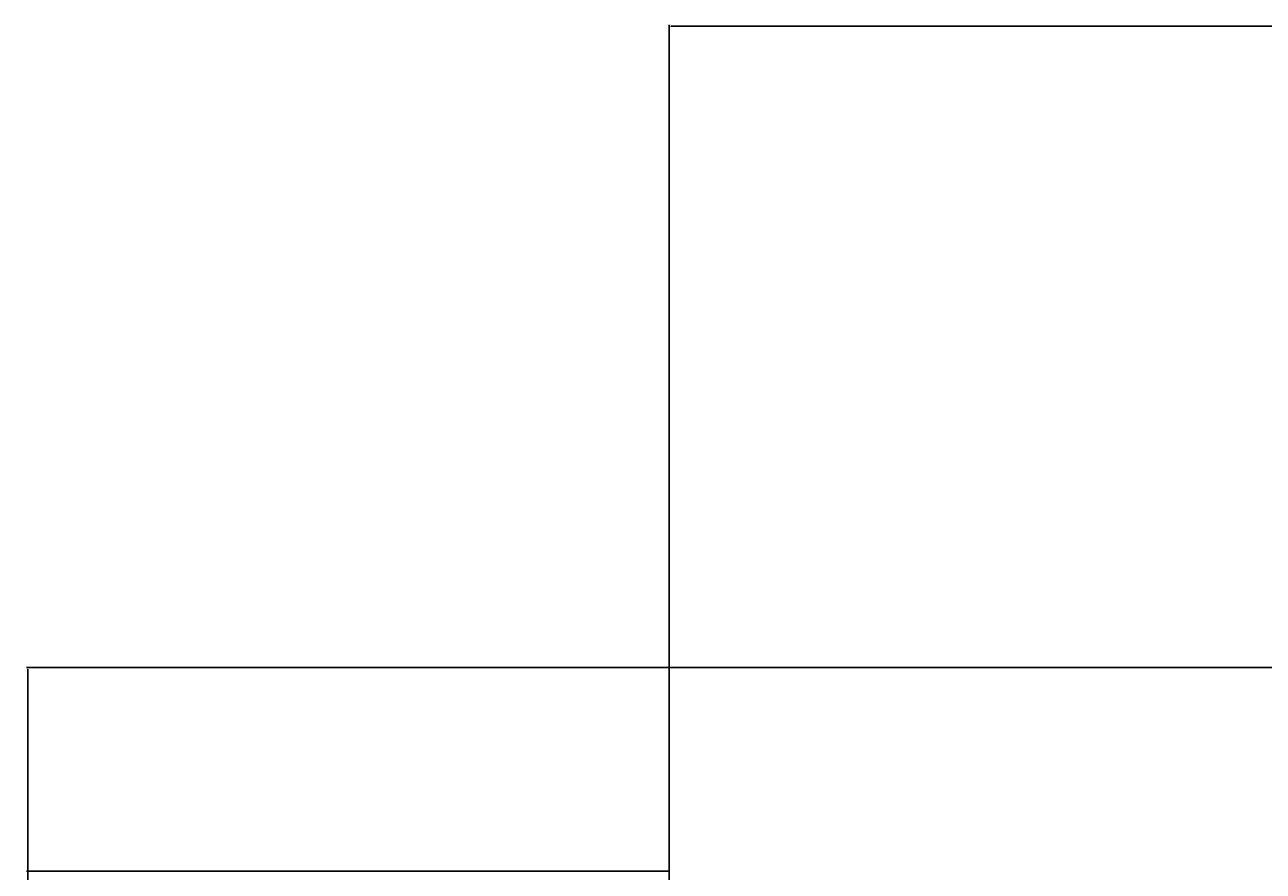
# Model space of a CAD drawing. Units: inches. Extents: x -61 to 1599, y -1316 to 257.
# Tile 113 of 204: x -61 to 85, y 158 to 257. Entities that reach past the tile are written whole.
import ezdxf

# ---------------------------------------------------------------- set-up
doc = ezdxf.new("R2010")
doc.units = ezdxf.units.IN
doc.header["$MEASUREMENT"] = 0
doc.layers.add('A-ANNO-DIMS', color=2, linetype='Continuous', lineweight=18)
doc.styles.get("Standard").update_dxf_attribs({"font": 'arial.ttf'})
doc.dimstyles.get("Standard").update_dxf_attribs({"dimtxt": 0.18, "dimasz": 0.18, "dimexe": 0.18, "dimexo": 0.0625, "dimgap": 0.09, "dimtad": 0, "dimtih": 1, "dimtoh": 1, "dimdec": 0, "dimzin": 0, "dimdsep": 46, "dimlunit": 3, "dimtxsty": 'Standard', "dimcen": 0.09, "dimadec": 0, "dimazin": 0, "dimtfac": 1, "dimtdec": 0, "dimtofl": 0, "dimtmove": 0, "dimatfit": 3, "dimfxl": 1, "dimtolj": 1, "dimtzin": 0, "dimarcsym": 0})

# ---------------------------------------------------------------- blocks, each defined once
blk = doc.blocks.new('*D686')
at = {"layer": 'A-ANNO-DIMS', "color": 0, "lineweight": -2, "transparency": 16777216}
for p, q in [((14.7, 157.74), (14.7, 257.46)), ((14.88, 257.28), (768.35, 257.28)), ((1522.52, 257.28), (769.05, 257.28)), ((1522.7, 157.74), (1522.7, 257.46))]:
    blk.add_line(p, q, dxfattribs=at)
at = {"layer": 'A-ANNO-DIMS', "color": 0, "transparency": 16777216}
for points in [[(14.88, 257.31), (14.88, 257.25), (14.7, 257.28)], [(1522.52, 257.31), (1522.52, 257.25), (1522.7, 257.28)]]:
    blk.add_solid(points, dxfattribs=at)
at = {"layer": 'DEFPOINTS', "color": 0, "transparency": 16777216}
for p in [(1522.7, 257.28), (14.7, 157.68), (1522.7, 157.68)]:
    blk.add_point(p, dxfattribs=at)
at = {"layer": 'A-ANNO-DIMS', "color": 0, "transparency": 16777216, "insert": (768.7, 257.28), "char_height": 0.18, "attachment_point": 5}
blk.add_mtext('\\A1;1508', dxfattribs=at)
blk = doc.blocks.new('*D687')
at = {"layer": 'A-ANNO-DIMS', "color": 0, "lineweight": -2, "transparency": 16777216}
for p, q in [((289.42, 181.68), (-61.08, 181.68)), ((-60.9, 181.5), (-60.9, -528.95)), ((-60.9, -1239.76), (-60.9, -529.32)), ((319.64, -1239.94), (-61.08, -1239.94))]:
    blk.add_line(p, q, dxfattribs=at)
at = {"layer": 'A-ANNO-DIMS', "color": 0, "transparency": 16777216}
for points in [[(-60.93, 181.5), (-60.87, 181.5), (-60.9, 181.68)], [(-60.93, -1239.76), (-60.87, -1239.76), (-60.9, -1239.94)]]:
    blk.add_solid(points, dxfattribs=at)
at = {"layer": 'DEFPOINTS', "color": 0, "transparency": 16777216}
for p in [(289.48, 181.68), (-60.9, -1239.94), (319.7, -1239.94)]:
    blk.add_point(p, dxfattribs=at)
at = {"layer": 'A-ANNO-DIMS', "color": 0, "transparency": 16777216, "insert": (-60.9, -529.13), "char_height": 0.18, "attachment_point": 5}
blk.add_mtext('\\A1;1421.6', dxfattribs=at)
blk = doc.blocks.new('*D691')
at = {"layer": 'A-ANNO-DIMS', "color": 0, "lineweight": -2, "transparency": 16777216}
for p, q in [((14.64, 157.68), (-61.08, 157.68)), ((-60.9, 157.5), (-60.9, -141.64)), ((-60.9, -441.14), (-60.9, -142)), ((14.64, -441.32), (-61.08, -441.32))]:
    blk.add_line(p, q, dxfattribs=at)
at = {"layer": 'A-ANNO-DIMS', "color": 0, "transparency": 16777216}
for points in [[(-60.93, 157.5), (-60.87, 157.5), (-60.9, 157.68)], [(-60.93, -441.14), (-60.87, -441.14), (-60.9, -441.32)]]:
    blk.add_solid(points, dxfattribs=at)
at = {"layer": 'DEFPOINTS', "color": 0, "transparency": 16777216}
for p in [(-60.9, 157.68), (14.7, 157.68), (14.7, -441.32)]:
    blk.add_point(p, dxfattribs=at)
at = {"layer": 'A-ANNO-DIMS', "color": 0, "transparency": 16777216, "insert": (-60.9, -141.82), "char_height": 0.18, "attachment_point": 5}
blk.add_mtext('\\A1;599', dxfattribs=at)
blk = doc.blocks.new('*D700')
at = {"layer": 'A-ANNO-DIMS', "color": 0, "lineweight": -2, "transparency": 16777216}
for p, q in [((14.7, -616.88), (14.7, 257.46)), ((14.88, 257.28), (96.77, 257.28)), ((179.57, 257.28), (97.68, 257.28)), ((179.75, -616.88), (179.75, 257.46))]:
    blk.add_line(p, q, dxfattribs=at)
at = {"layer": 'A-ANNO-DIMS', "color": 0, "transparency": 16777216}
for points in [[(14.88, 257.31), (14.88, 257.25), (14.7, 257.28)], [(179.57, 257.31), (179.57, 257.25), (179.75, 257.28)]]:
    blk.add_solid(points, dxfattribs=at)
at = {"layer": 'DEFPOINTS', "color": 0, "transparency": 16777216}
for p in [(179.75, 257.28), (14.7, -616.94), (179.75, -616.94)]:
    blk.add_point(p, dxfattribs=at)
at = {"layer": 'A-ANNO-DIMS', "color": 0, "transparency": 16777216, "insert": (97.23, 257.28), "char_height": 0.18, "attachment_point": 5}
blk.add_mtext('\\A1;165.05', dxfattribs=at)

msp = doc.modelspace()

# ---------------------------------------------------------------- dimensions: what is measured, and where the dimension line sits
at = {"layer": 'A-ANNO-DIMS'}
for base, p1, p2, override, picture, middle in [((1522.7028, 257.2771), (14.7028, 157.6771), (1522.7028, 157.6771), {"dimdec": 0, "dimlfac": 1, "dimrnd": 0, "dimzin": 0, "dimdsep": 46, "dimlunit": 2}, '*D686', (768.7028, 257.2771)), ((179.7521, 257.2771), (14.7028, -616.9446), (179.7521, -616.9446), {"dimdec": 2, "dimlfac": 1, "dimrnd": 0, "dimzin": 0, "dimdsep": 46, "dimlunit": 2}, '*D700', (97.2274, 257.2771))]:
    dim = msp.add_linear_dim(base=base, p1=p1, p2=p2, dimstyle='Standard', override=override, dxfattribs=at)
    dim.commit()
    dim.dimension.update_dxf_attribs({"geometry": picture, "text_midpoint": middle})
for base, p1, p2, override, picture, middle in [((-60.8972, -1239.9446), (289.4807, 181.6771), (319.7028, -1239.9446), {"dimdec": 1, "dimlfac": 1, "dimrnd": 0, "dimzin": 0, "dimdsep": 46, "dimlunit": 2}, '*D687', (-60.8972, -529.1337)), ((-60.8972, 157.6771), (14.7028, -441.3229), (14.7028, 157.6771), {"dimdec": 0, "dimlfac": 1, "dimrnd": 0, "dimzin": 0, "dimdsep": 46, "dimlunit": 2}, '*D691', (-60.8972, -141.8229))]:
    dim = msp.add_linear_dim(base=base, p1=p1, p2=p2, angle=90, dimstyle='Standard', override=override, dxfattribs=at)
    dim.commit()
    dim.dimension.update_dxf_attribs({"geometry": picture, "text_midpoint": middle})

doc.saveas('drawing.dxf')
